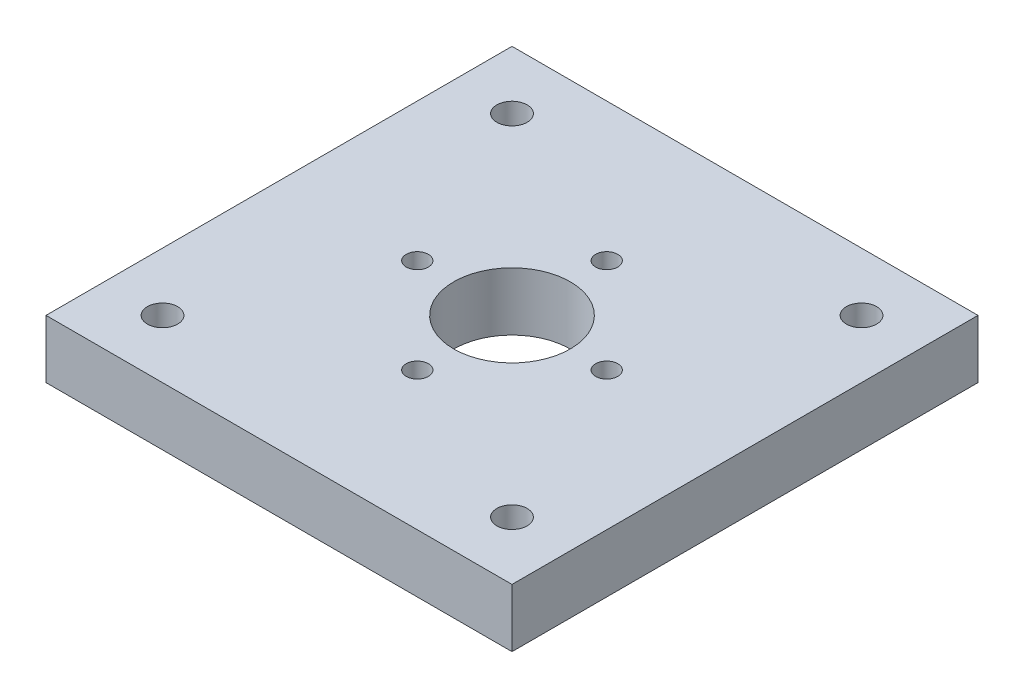
from build123d import *

# Parameters (mm, degrees)
BASE_PLATE_PROFILE_W        = 400
BASE_PLATE_PROFILE_H        = 400
BASE_PLATE_PROFILE_R        = 50
BASE_PLATE_PROFILE_R_2      = 13
BASE_PLATE_PROFILE_R_3      = 9.5
BASE_PLATE_400X400X50_DEPTH = 25


with BuildPart() as part:
    # Base Plate Profile → Base Plate 400x400x50 (new, symmetric)
    with BuildSketch(Plane(origin=(0, 0, 0), x_dir=(1, 0, 0), z_dir=(0, 1, 0))):
        Rectangle(BASE_PLATE_PROFILE_W, BASE_PLATE_PROFILE_H)
        with Locations(Location((0, 0, 0), (0, 0, 270))):
            Circle(BASE_PLATE_PROFILE_R, mode=Mode.SUBTRACT)
        with Locations(Location((150, 150, 0), (0, 0, 270))):
            Circle(BASE_PLATE_PROFILE_R_2, mode=Mode.SUBTRACT)
        with Locations(Location((-150, 150, 0), (0, 0, 90))):
            Circle(BASE_PLATE_PROFILE_R_2, mode=Mode.SUBTRACT)
        with Locations(Location((150, -150, 0), (0, 0, 90))):
            Circle(BASE_PLATE_PROFILE_R_2, mode=Mode.SUBTRACT)
        with Locations(Location((-150, -150, 0), (0, 0, 270))):
            Circle(BASE_PLATE_PROFILE_R_2, mode=Mode.SUBTRACT)
        with Locations(Location((0, 81.3, 0), (0, 0, 270))):
            Circle(BASE_PLATE_PROFILE_R_3, mode=Mode.SUBTRACT)
        with Locations(Location((0, -81.3, 0), (0, 0, 90))):
            Circle(BASE_PLATE_PROFILE_R_3, mode=Mode.SUBTRACT)
        with Locations(Location((-81.3, 0, 0), (0, 0, 270))):
            Circle(BASE_PLATE_PROFILE_R_3, mode=Mode.SUBTRACT)
        with Locations(Location((81.3, 0, 0), (0, 0, 90))):
            Circle(BASE_PLATE_PROFILE_R_3, mode=Mode.SUBTRACT)
    extrude(amount=BASE_PLATE_400X400X50_DEPTH, both=True)


solid = part.part
